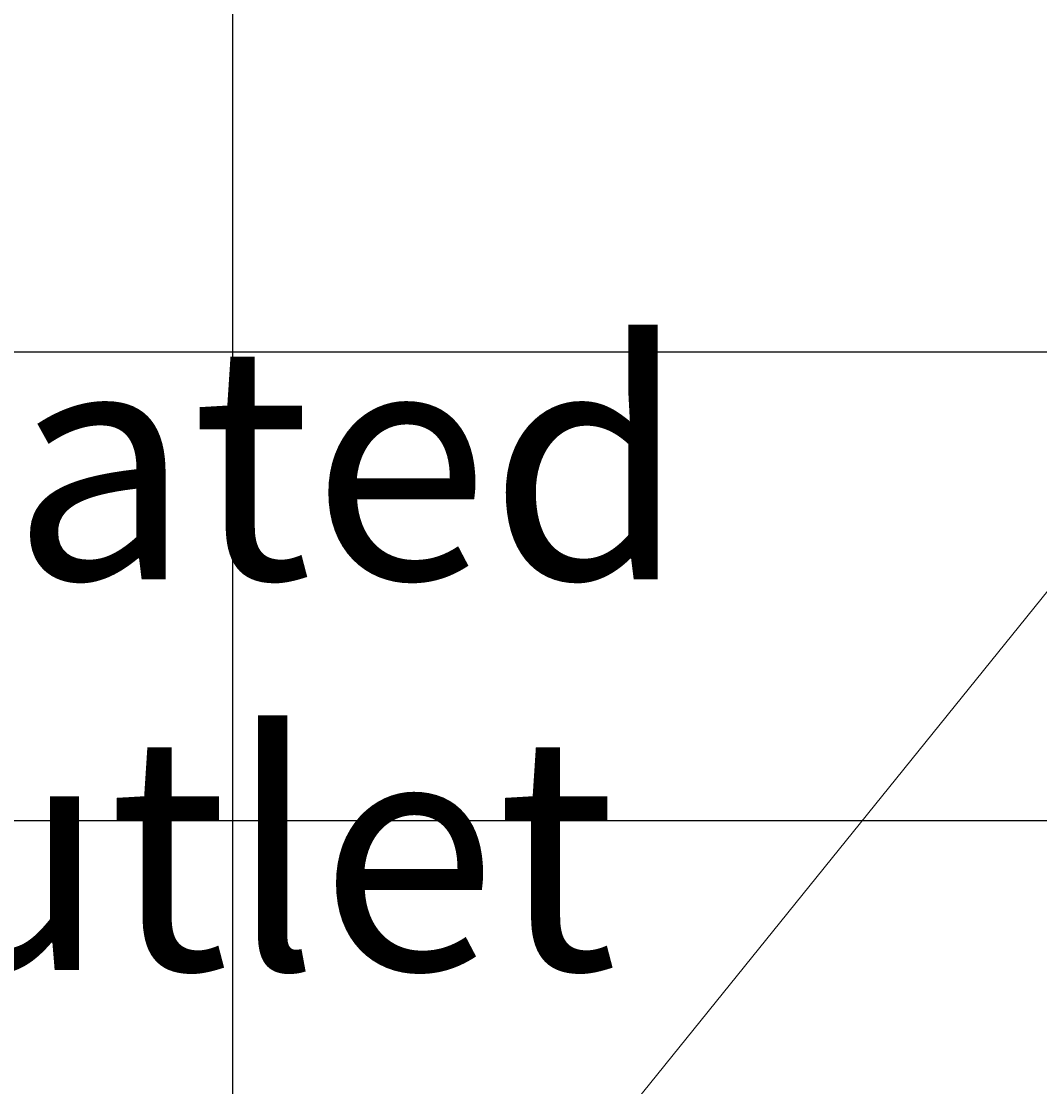
# Model space of a CAD drawing. Units: inches. Extents: x -1 to 292, y -3 to 199.
# Tile 35 of 52: x 210.74 to 232.46, y 19.84 to 42.57. Entities that reach past the tile are written whole.
import ezdxf

# ---------------------------------------------------------------- set-up
doc = ezdxf.new("R2010")
doc.units = ezdxf.units.IN
doc.header["$MEASUREMENT"] = 0
for name, color, linetype, lineweight in [('M-ANNO-LEAD', 2, 'Continuous', 18), ('M-ANNO-TEXT', 3, 'Continuous', 25), ('M-DIMS', 2, 'Continuous', 18)]:
    doc.layers.add(name, color=color, linetype=linetype, lineweight=lineweight)
doc.styles.get("Standard").update_dxf_attribs({"font": 'arial.ttf'})
doc.dimstyles.get("Standard").update_dxf_attribs({"dimtxt": 0.18, "dimasz": 0.18, "dimexe": 0.18, "dimexo": 0.0625, "dimgap": 0.09, "dimtad": 0, "dimtih": 1, "dimtoh": 1, "dimdec": 4, "dimzin": 0, "dimdsep": 46, "dimtxsty": 'Standard', "dimcen": 0.09, "dimadec": 0, "dimazin": 0, "dimtfac": 1, "dimtdec": 4, "dimtofl": 0, "dimtmove": 0, "dimatfit": 3, "dimfxl": 1, "dimtolj": 1, "dimtzin": 0, "dimarcsym": 0})

# ---------------------------------------------------------------- blocks, each defined once
blk = doc.blocks.new('*D11')
at = {"layer": 'Defpoints', "color": 0, "transparency": 16777216}
for p in [(79.013, 35.514), (292.04, 35.514), (79.013, 25.514)]:
    blk.add_point(p, dxfattribs=at)
at = {"layer": 'M-DIMS', "color": 0, "lineweight": -2, "transparency": 16777216}
for p, q in [((79.076, 35.514), (292.22, 35.514)), ((292.04, 35.334), (292.04, 30.696)), ((292.04, 25.694), (292.04, 30.332)), ((79.076, 25.514), (292.22, 25.514))]:
    blk.add_line(p, q, dxfattribs=at)
at = {"layer": 'M-DIMS', "color": 0, "transparency": 16777216}
for points in [[(292.01, 35.334), (292.07, 35.334), (292.04, 35.514)], [(292.01, 25.694), (292.07, 25.694), (292.04, 25.514)]]:
    blk.add_solid(points, dxfattribs=at)
at = {"layer": 'M-DIMS', "color": 0, "transparency": 16777216, "insert": (292.04, 30.514), "char_height": 0.18, "attachment_point": 5}
blk.add_mtext('\\A1;10', dxfattribs=at)
blk = doc.blocks.new('*D24')
at = {"layer": 'Defpoints', "color": 0, "transparency": 16777216}
for p in [(215.241, 55.034), (205.115, 54.582), (215.241, -2.71)]:
    blk.add_point(p, dxfattribs=at)
at = {"layer": 'M-DIMS', "color": 0, "lineweight": -2, "transparency": 16777216}
for p, q in [((215.241, 54.971), (215.241, -2.89)), ((205.115, 54.52), (205.115, -2.89)), ((205.295, -2.71), (209.722, -2.71)), ((215.061, -2.71), (210.634, -2.71))]:
    blk.add_line(p, q, dxfattribs=at)
at = {"layer": 'M-DIMS', "color": 0, "transparency": 16777216}
for points in [[(205.295, -2.68), (205.295, -2.74), (205.115, -2.71)], [(215.061, -2.68), (215.061, -2.74), (215.241, -2.71)]]:
    blk.add_solid(points, dxfattribs=at)
at = {"layer": 'M-DIMS', "color": 0, "transparency": 16777216, "insert": (210.178, -2.71), "char_height": 0.18, "attachment_point": 5}
blk.add_mtext('\\A1;10.125', dxfattribs=at)
blk = doc.blocks.new('*D25')
at = {"layer": 'Defpoints', "color": 0, "transparency": 16777216}
for p in [(273.066, 88.419), (215.241, 88.13), (273.066, -2.71)]:
    blk.add_point(p, dxfattribs=at)
at = {"layer": 'M-DIMS', "color": 0, "lineweight": -2, "transparency": 16777216}
for p, q in [((273.066, 88.357), (273.066, -2.89)), ((215.241, 88.068), (215.241, -2.89)), ((215.421, -2.71), (243.76, -2.71)), ((272.886, -2.71), (244.547, -2.71))]:
    blk.add_line(p, q, dxfattribs=at)
at = {"layer": 'M-DIMS', "color": 0, "transparency": 16777216}
for points in [[(215.421, -2.68), (215.421, -2.74), (215.241, -2.71)], [(272.886, -2.68), (272.886, -2.74), (273.066, -2.71)]]:
    blk.add_solid(points, dxfattribs=at)
at = {"layer": 'M-DIMS', "color": 0, "transparency": 16777216, "insert": (244.153, -2.71), "char_height": 0.18, "attachment_point": 5}
blk.add_mtext('\\A1;57.83', dxfattribs=at)

msp = doc.modelspace()

# ---------------------------------------------------------------- linework, layer by layer
at = {"layer": 'M-ANNO-LEAD'}
msp.add_line((239.9895, 39.5261), (217.6733, 11.8896), dxfattribs=at)

# ---------------------------------------------------------------- texts
at = {"layer": 'M-ANNO-TEXT', "insert": (183.0839, 35.6644), "char_height": 5, "attachment_point": 1}
msp.add_mtext_dynamic_manual_height_columns('super heated steam outlet', width=47.899539, gutter_width=1, heights=[0], dxfattribs=at)

# ---------------------------------------------------------------- dimensions: what is measured, and where the dimension line sits
at = {"layer": 'M-DIMS'}
for base, p1, p2, override, picture, middle in [((273.0659, -2.7104), (215.2407, 88.1304), (273.0659, 88.4191), {"dimdec": 2, "dimlfac": 1, "dimrnd": 0, "dimzin": 0, "dimdsep": 46, "dimlunit": 2}, '*D25', (244.1533, -2.7104)), ((215.2407, -2.7104), (205.1155, 54.5821), (215.2407, 55.0337), {"dimdec": 3, "dimlfac": 1, "dimrnd": 0, "dimzin": 0, "dimdsep": 46, "dimlunit": 2}, '*D24', (210.1781, -2.7104))]:
    dim = msp.add_linear_dim(base=base, p1=p1, p2=p2, dimstyle='Standard', override=override, dxfattribs=at)
    dim.commit()
    dim.dimension.update_dxf_attribs({"geometry": picture, "text_midpoint": middle})
dim = msp.add_linear_dim(base=(292.0399, 35.5141), p1=(79.013, 25.5141), p2=(79.013, 35.5141), angle=90, dimstyle='Standard', override={"dimdec": 0, "dimlfac": 1, "dimrnd": 0, "dimzin": 0, "dimdsep": 46, "dimlunit": 2}, dxfattribs=at)
dim.commit()
dim.dimension.update_dxf_attribs({"geometry": '*D11', "text_midpoint": (292.0399, 30.5141)})

doc.saveas('drawing.dxf')
